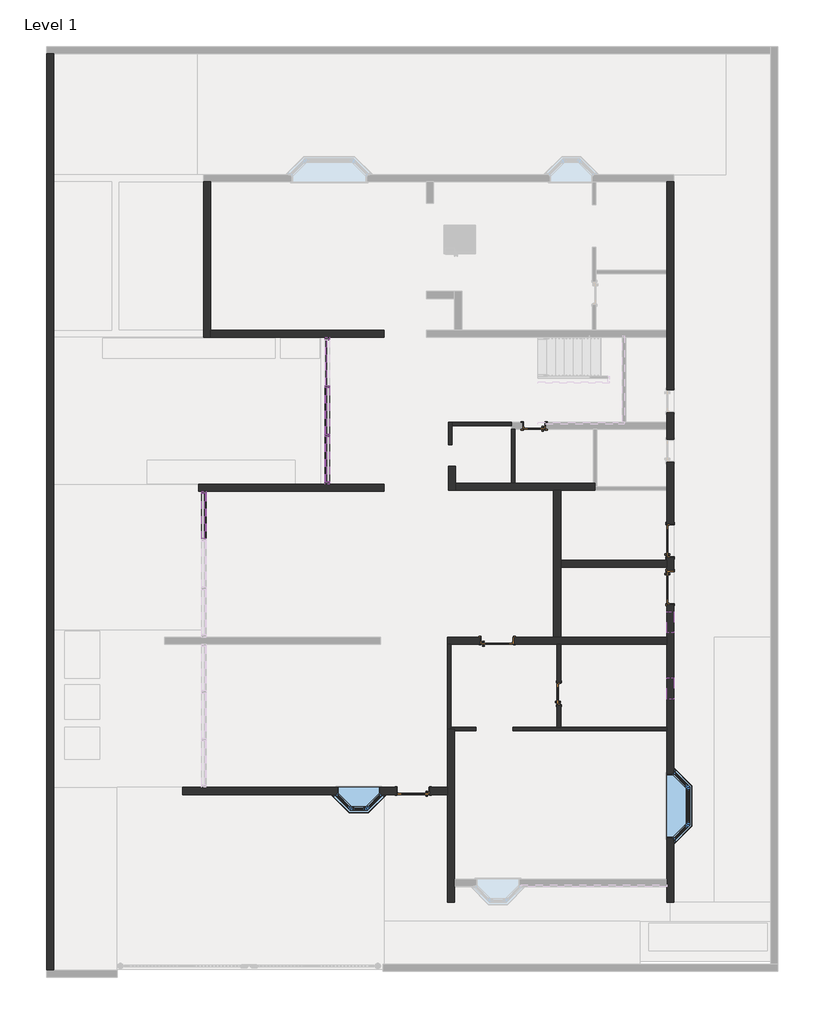
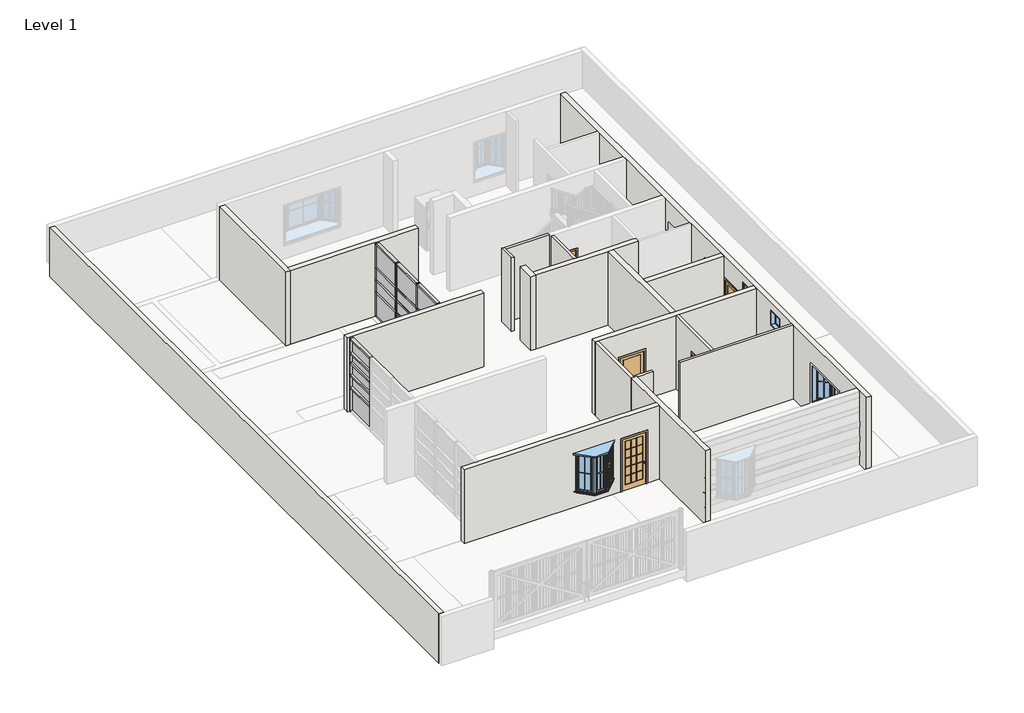
# One storey, part 3 of 5: 38 members, 19 walls, 17 plates, 6 doors, 4 windows.
# Revit data of these elements (continued)
# Element 80 (IfcWall, "OUTER WALL 8\"") (continued)
#   Base Offset = -1' - 7.86555"
#   Unconnected Height = 6' - 7.86555"
#   wall height = 6' - 7.86555"
#   Phase Created = New Construction
#   Base Constraint = Level 1
#   Materials on its faces: "BEIGE COLOUR"
# Element 81 (IfcWindow, "Fixed : 24\" x 24\"")
#   Mark = "5"
#   Phase Created = New Construction
#   Materials on its faces: "Sash", "Glass"
# Element 82 (IfcWindow, "Fixed : 24\" x 24\"")
#   Mark = "6"
#   Phase Created = New Construction
#   Materials on its faces: "Sash", "Glass"
# Element 83 (IfcWindow, "Window-Bay-Casement-45_Degree_Angle : WINDOW 4'")
#   Mark = "7"
#   Interior Trim Visibility = yes
#   Exterior Trim Visibility = yes
#   Phase Created = New Construction
#   Materials on its faces: "Wood - Stained", "Clad - White", "Glass"
# Element 84 (IfcWindow, "Window-Bay-Casement-45_Degree_Angle : WINDOW 6'X4'")
#   Mark = "4"
#   Interior Trim Visibility = yes
#   Exterior Trim Visibility = yes
#   Phase Created = New Construction
#   Materials on its faces: "Wood - Stained", "Clad - White", "Glass"
# Materials
#   "Cherry": class "Wood", colour RGB 226 177 128, transparency 0, Description = "Prunus Serotina", Cost = 0
#   "Aluminum": class "Metal", colour RGB 247 247 247, transparency 0, Description = "Aluminum 6061", Cost = 0
#   "BEIGE COLOUR": class "Generic", colour RGB 120 120 120, transparency 0, Cost = 0
#   "Glass": class "Glass", colour RGB 0 128 192, transparency 0.75, Description = "Soda Lime Glass", Cost = 0
#   "Sash": class "Wood", colour RGB 224 178 126, transparency 0, Cost = 0
#   "Wood - Stained": class "Wood", colour RGB 224 178 126, transparency 0, Cost = 0
#   "Clad - White": class "Wood", colour RGB 242 242 238, transparency 0, Cost = 0
#   "glass panel 223": class "Generic", colour RGB 120 120 120, transparency 0, Cost = 0
